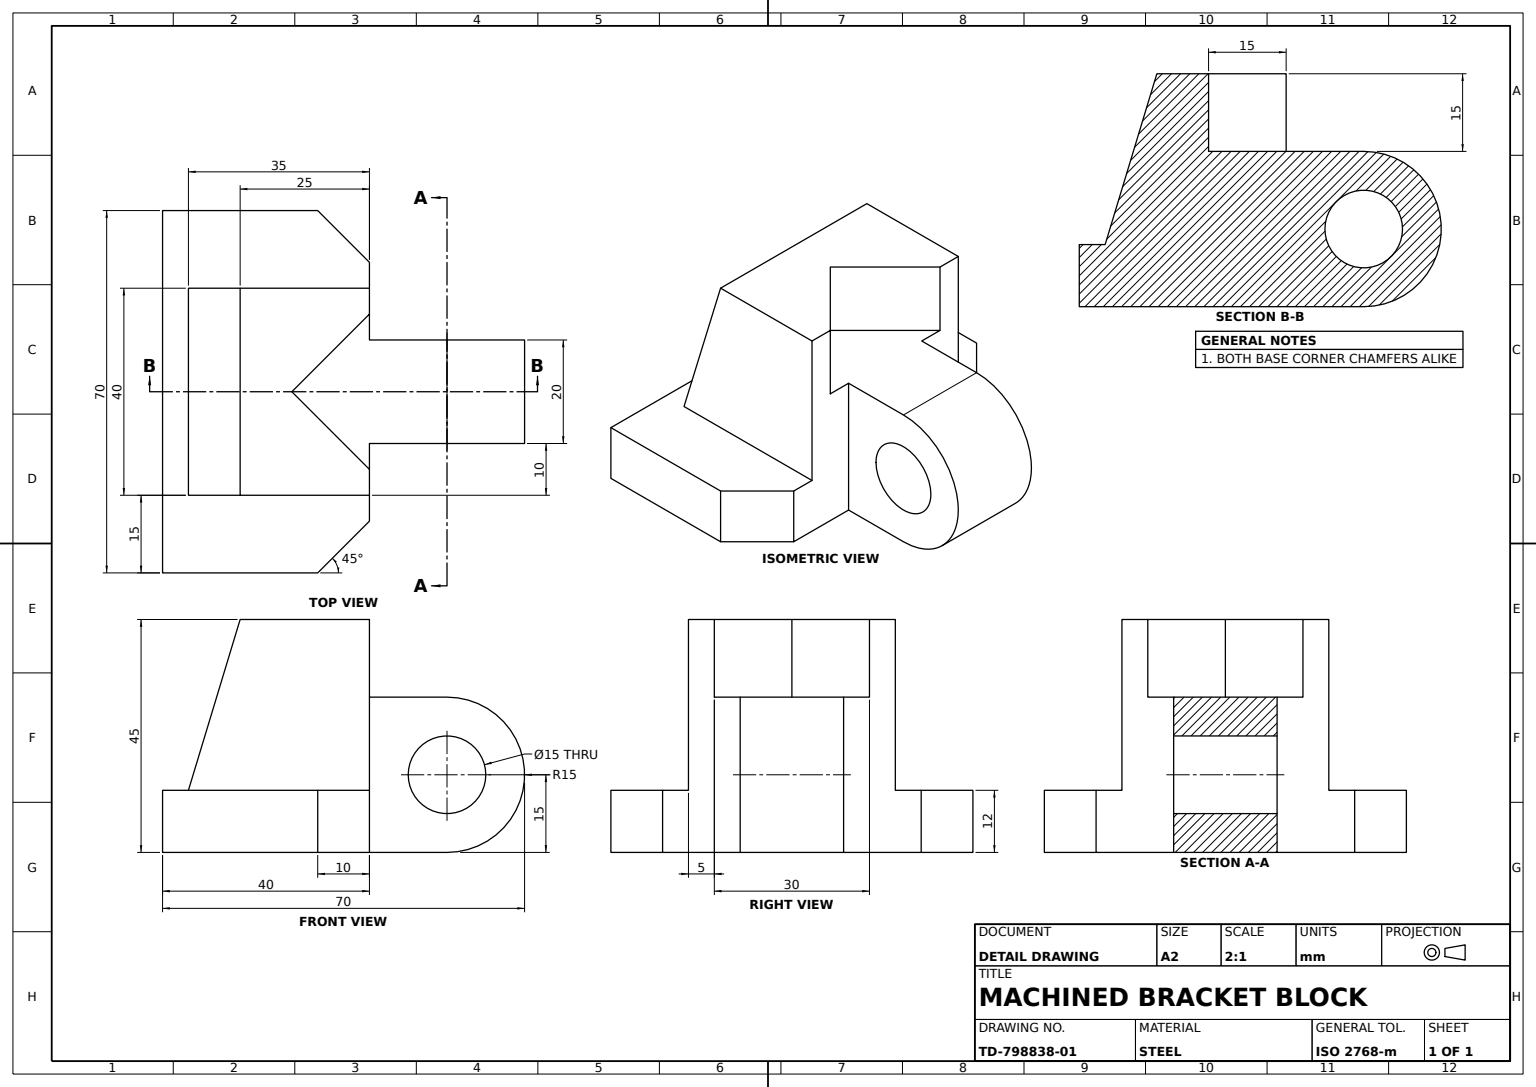
from build123d import *

# Parameters (mm, degrees)
BRACKET_PROFILE_SKETCH_R       = 7.5
LUG_EYE_BOSS_20MM_DEPTH        = 10
SKETCH5_3_W                    = 40
SKETCH5_3_H                    = 12
BASE_BLOCK_70MM_DEPTH          = 35
UPRIGHT_BLOCK_40MM_DEPTH       = 20
UPRIGHT_EDGE_CHAMFER_10MM_SIZE = 10
FORK_SLOT_CUT_30X15_DEPTH      = 15


with BuildPart() as part:
    # Bracket Profile Sketch → Lug Eye Boss 20mm (new, symmetric)
    with BuildSketch(Plane.XY):
        with BuildLine():
            Line((-15, -3), (-15, -15))
            Line((-15, -15), (0, -15))
            ThreePointArc((0, -15), (15, 0), (0, 15))
            Line((0, 15), (-15, 15))
            Line((-15, 15), (-15, -3))
        make_face()
        Circle(BRACKET_PROFILE_SKETCH_R, mode=Mode.SUBTRACT)
    extrude(amount=LUG_EYE_BOSS_20MM_DEPTH, both=True)

    # Sketch5_3 → Base Block 70mm (add, symmetric)
    with BuildSketch(Plane.XY):
        with Locations((-35, -9)):
            Rectangle(SKETCH5_3_W, SKETCH5_3_H)
    extrude(amount=BASE_BLOCK_70MM_DEPTH, both=True)

    # Sketch5_4 → Upright Block 40mm (add, symmetric)
    with BuildSketch(Plane.XY):
        Polygon((-50, -3), (-15, -3), (-15, 15), (-15, 30), (-40, 30), align=None)
    extrude(amount=UPRIGHT_BLOCK_40MM_DEPTH, both=True)

    # Upright Edge Chamfer 10mm
    upright_edge_chamfer_10mm_edges = [part.edges().sort_by_distance(p)[0] for p in [
        (-15, -9, -35),
        (-15, -9, 35),
    ]]
    chamfer(upright_edge_chamfer_10mm_edges, length=UPRIGHT_EDGE_CHAMFER_10MM_SIZE)

    # Fork Slot Sketch → Fork Slot Cut 30x15 (cut)
    with BuildSketch(Plane(origin=(0, 30, 0), x_dir=(1, 0, 0), z_dir=(0, 1, 0))):
        Polygon((-15, -15), (-30, 0), (-15, 15), align=None)
    extrude(amount=-FORK_SLOT_CUT_30X15_DEPTH, mode=Mode.SUBTRACT)


solid = part.part
